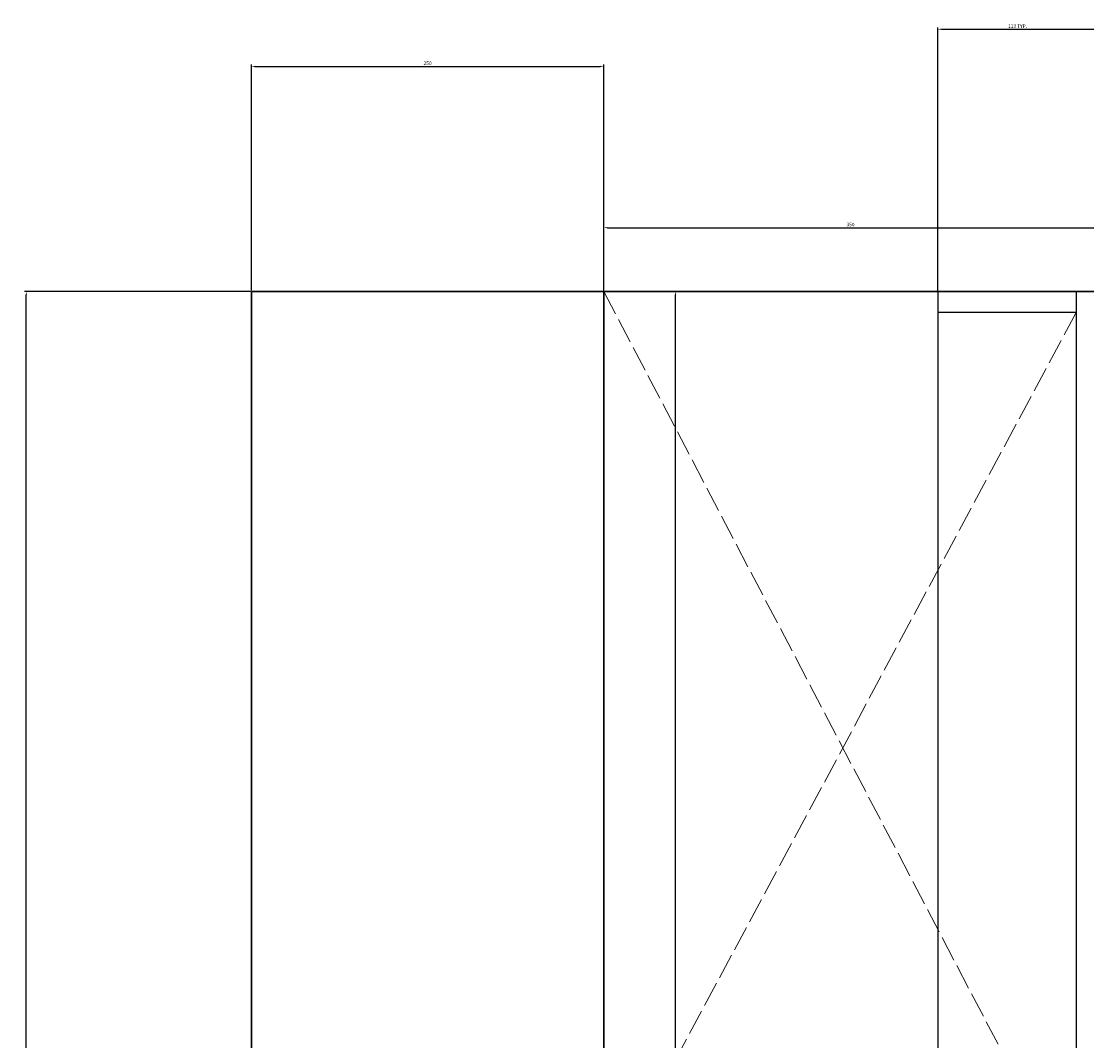
# Model space of a CAD drawing. Units: millimetres. Extents: x 2332 to 5836, y -853 to 2199.
# Tile 5 of 16: x 2332 to 3088, y 1476 to 2199. Entities that reach past the tile are written whole.
import ezdxf

# ---------------------------------------------------------------- set-up
doc = ezdxf.new("R2010")
doc.units = ezdxf.units.MM
doc.linetypes.add('ACAD_ISO02W100', pattern=[15, 12, -3])
doc.layers.get('0').update_dxf_attribs({"color": 8})
for name, color, linetype, lineweight in [('A-ANNO-DIMS', 2, 'Continuous', 18), ('A-CSWK-HIDN', 8, 'ACAD_ISO02W100', 13), ('A-WALL', 8, 'Continuous', 30), ('SHELF', 40, 'Continuous', 25)]:
    doc.layers.add(name, color=color, linetype=linetype, lineweight=lineweight)
doc.styles.get("Standard").update_dxf_attribs({"font": 'arial.ttf'})
doc.dimstyles.new('ISO-25', dxfattribs={"dimtxt": 2.5, "dimasz": 2.5, "dimexe": 1.25, "dimexo": 0.625, "dimtad": 1, "dimtxsty": 'Standard', "dimcen": 2.5, "dimadec": 0, "dimazin": 0, "dimtfac": 1, "dimtmove": 0, "dimatfit": 3, "dimfxl": 1, "dimarcsym": 0})

# ---------------------------------------------------------------- blocks, each defined once
blk = doc.blocks.new('*D1')
at = {"layer": 'A-ANNO-DIMS', "color": 0, "lineweight": -2, "transparency": 16777216}
for p, q in [((2745.04, 2008.43), (2745.04, 2054.25)), ((2747.54, 2053), (3092.54, 2053)), ((3095.04, 2008.43), (3095.04, 2054.25))]:
    blk.add_line(p, q, dxfattribs=at)
at = {"layer": 'A-ANNO-DIMS', "color": 0, "transparency": 16777216}
for points in [[(2747.54, 2053.41), (2747.54, 2052.58), (2745.04, 2053)], [(3092.54, 2053.41), (3092.54, 2052.58), (3095.04, 2053)]]:
    blk.add_solid(points, dxfattribs=at)
at = {"layer": 'Defpoints', "color": 0, "transparency": 16777216}
for p in [(3095.04, 2053), (2745.04, 2007.8), (3095.04, 2007.8)]:
    blk.add_point(p, dxfattribs=at)
at = {"layer": 'A-ANNO-DIMS', "color": 0, "transparency": 16777216, "insert": (2920.04, 2054.9), "char_height": 2.5, "attachment_point": 5}
blk.add_mtext('350', dxfattribs=at)
blk = doc.blocks.new('CAB-END-STILE')
for p, q in [((0, 1240), (0, 600)), ((98.09, 1240), (98.09, 0)), ((98.09, 1225), (0, 1225))]:
    blk.add_line(p, q)
blk = doc.blocks.new('*D11')
at = {"layer": 'A-ANNO-DIMS', "color": 0, "lineweight": -2, "transparency": 16777216}
for p, q in [((2981.33, 2007.8), (2794.7, 2007.8)), ((2795.95, 770.3), (2795.95, 2005.3)), ((2981.33, 767.8), (2794.7, 767.8))]:
    blk.add_line(p, q, dxfattribs=at)
at = {"layer": 'A-ANNO-DIMS', "color": 0, "transparency": 16777216}
for points in [[(2795.53, 2005.3), (2796.37, 2005.3), (2795.95, 2007.8)], [(2795.53, 770.3), (2796.37, 770.3), (2795.95, 767.8)]]:
    blk.add_solid(points, dxfattribs=at)
at = {"layer": 'Defpoints', "color": 0, "transparency": 16777216}
for p in [(2795.95, 2007.8), (2981.95, 2007.8), (2981.95, 767.8)]:
    blk.add_point(p, dxfattribs=at)
at = {"layer": 'A-ANNO-DIMS', "color": 0, "transparency": 16777216, "insert": (2794.03, 1387.8), "char_height": 2.5, "attachment_point": 5, "rotation": 90}
blk.add_mtext('END STILE 1240 TYP.', dxfattribs=at)
blk = doc.blocks.new('*D12')
at = {"layer": 'A-ANNO-DIMS', "color": 0, "lineweight": -2, "transparency": 16777216}
for p, q in [((2981.95, 2008.43), (2981.95, 2195.05)), ((2984.45, 2193.8), (3092.54, 2193.8)), ((3095.04, 2008.43), (3095.04, 2195.05))]:
    blk.add_line(p, q, dxfattribs=at)
at = {"layer": 'A-ANNO-DIMS', "color": 0, "transparency": 16777216}
for points in [[(2984.45, 2194.22), (2984.45, 2193.39), (2981.95, 2193.8)], [(3092.54, 2194.22), (3092.54, 2193.39), (3095.04, 2193.8)]]:
    blk.add_solid(points, dxfattribs=at)
at = {"layer": 'Defpoints', "color": 0, "transparency": 16777216}
for p in [(3095.04, 2193.8), (2981.95, 2007.8), (3095.04, 2007.8)]:
    blk.add_point(p, dxfattribs=at)
at = {"layer": 'A-ANNO-DIMS', "color": 0, "transparency": 16777216, "insert": (3038.49, 2195.71), "char_height": 2.5, "attachment_point": 5}
blk.add_mtext('113 TYP.', dxfattribs=at)
blk = doc.blocks.new('*D16')
at = {"layer": 'A-ANNO-DIMS', "color": 0, "lineweight": -2, "transparency": 16777216}
for p, q in [((2494.41, 2007.8), (2334.14, 2007.8)), ((2335.39, -689.7), (2335.39, 2005.3)), ((2494.41, -692.2), (2334.14, -692.2))]:
    blk.add_line(p, q, dxfattribs=at)
at = {"layer": 'A-ANNO-DIMS', "color": 0, "transparency": 16777216}
for points in [[(2334.97, 2005.3), (2335.81, 2005.3), (2335.39, 2007.8)], [(2334.97, -689.7), (2335.81, -689.7), (2335.39, -692.2)]]:
    blk.add_solid(points, dxfattribs=at)
at = {"layer": 'Defpoints', "color": 0, "transparency": 16777216}
for p in [(2335.39, 2007.8), (2495.04, 2007.8), (2495.04, -692.2)]:
    blk.add_point(p, dxfattribs=at)
at = {"layer": 'A-ANNO-DIMS', "color": 0, "transparency": 16777216, "insert": (2333.49, 657.8), "char_height": 2.5, "attachment_point": 5, "rotation": 90}
blk.add_mtext('2700', dxfattribs=at)
blk = doc.blocks.new('*D17')
at = {"layer": 'A-ANNO-DIMS', "color": 0, "lineweight": -2, "transparency": 16777216}
for p, q in [((2495.04, 2008.43), (2495.04, 2168.7)), ((2497.54, 2167.45), (2742.54, 2167.45)), ((2745.04, 2008.43), (2745.04, 2168.7))]:
    blk.add_line(p, q, dxfattribs=at)
at = {"layer": 'A-ANNO-DIMS', "color": 0, "transparency": 16777216}
for points in [[(2497.54, 2167.87), (2497.54, 2167.04), (2495.04, 2167.45)], [(2742.54, 2167.87), (2742.54, 2167.04), (2745.04, 2167.45)]]:
    blk.add_solid(points, dxfattribs=at)
at = {"layer": 'Defpoints', "color": 0, "transparency": 16777216}
for p in [(2745.04, 2167.45), (2495.04, 2007.8), (2745.04, 2007.8)]:
    blk.add_point(p, dxfattribs=at)
at = {"layer": 'A-ANNO-DIMS', "color": 0, "transparency": 16777216, "insert": (2620.04, 2169.35), "char_height": 2.5, "attachment_point": 5}
blk.add_mtext('250', dxfattribs=at)

msp = doc.modelspace()

# ---------------------------------------------------------------- linework, layer by layer
at = {"layer": 'A-CSWK-HIDN', "ltscale": 1.5}
for p, q in [((2745.04, 2007.803), (3080.04, 1367.803)), ((3080.04, 1992.803), (2745.04, 1367.803))]:
    msp.add_line(p, q, dxfattribs=at)
at = {"layer": 'A-WALL'}
for p, q in [((2495.04, 2007.803), (2745.04, 2007.803)), ((2495.04, -692.197), (2495.04, 2007.803)), ((2745.04, 2007.803), (3095.04, 2007.803)), ((2745.04, -692.197), (2745.04, 2007.803))]:
    msp.add_line(p, q, dxfattribs=at)

# ---------------------------------------------------------------- block references
at = {"layer": 'SHELF'}
msp.add_blockref('CAB-END-STILE', (2981.95, 767.803), dxfattribs=at)

# ---------------------------------------------------------------- dimensions: what is measured, and where the dimension line sits
at = {"layer": 'A-ANNO-DIMS'}
dim = msp.add_linear_dim(base=(3095.04, 2193.803), p1=(2981.95, 2007.803), p2=(3095.04, 2007.803), text='<> TYP.', dimstyle='ISO-25', override={"dimdec": 0, "dimlfac": 1, "dimrnd": 0, "dimzin": 0, "dimdsep": 46, "dimlunit": 2}, dxfattribs=at)
dim.commit()
dim.dimension.update_dxf_attribs({"geometry": '*D12', "text_midpoint": (3038.495, 2195.706)})
for base, p1, p2, override, picture, middle in [((2745.04, 2167.453), (2495.04, 2007.803), (2745.04, 2007.803), {"dimdec": 0, "dimlfac": 1, "dimrnd": 0, "dimzin": 0, "dimdsep": 46, "dimlunit": 2}, '*D17', (2620.04, 2169.355)), ((3095.04, 2052.998), (2745.04, 2007.803), (3095.04, 2007.803), {"dimclrd": 0, "dimclre": 0, "dimclrt": 0}, '*D1', (2920.04, 2054.9))]:
    dim = msp.add_linear_dim(base=base, p1=p1, p2=p2, dimstyle='ISO-25', override=override, dxfattribs=at)
    dim.commit()
    dim.dimension.update_dxf_attribs({"geometry": picture, "text_midpoint": middle})
dim = msp.add_linear_dim(base=(2335.39, 2007.803), p1=(2495.04, -692.197), p2=(2495.04, 2007.803), angle=90, dimstyle='ISO-25', override={"dimdec": 0, "dimlfac": 1, "dimrnd": 0, "dimzin": 0, "dimdsep": 46, "dimlunit": 2}, dxfattribs=at)
dim.commit()
dim.dimension.update_dxf_attribs({"geometry": '*D16', "text_midpoint": (2333.488, 657.803)})
dim = msp.add_linear_dim(base=(2795.95, 2007.803), p1=(2981.95, 767.803), p2=(2981.95, 2007.803), angle=90, text='END STILE <> TYP.', dimstyle='ISO-25', override={"dimdec": 0, "dimlfac": 1, "dimrnd": 0, "dimzin": 0, "dimdsep": 46, "dimlunit": 2}, dxfattribs=at)
dim.commit()
dim.dimension.update_dxf_attribs({"geometry": '*D11', "text_midpoint": (2794.032, 1387.803)})

doc.saveas('drawing.dxf')
